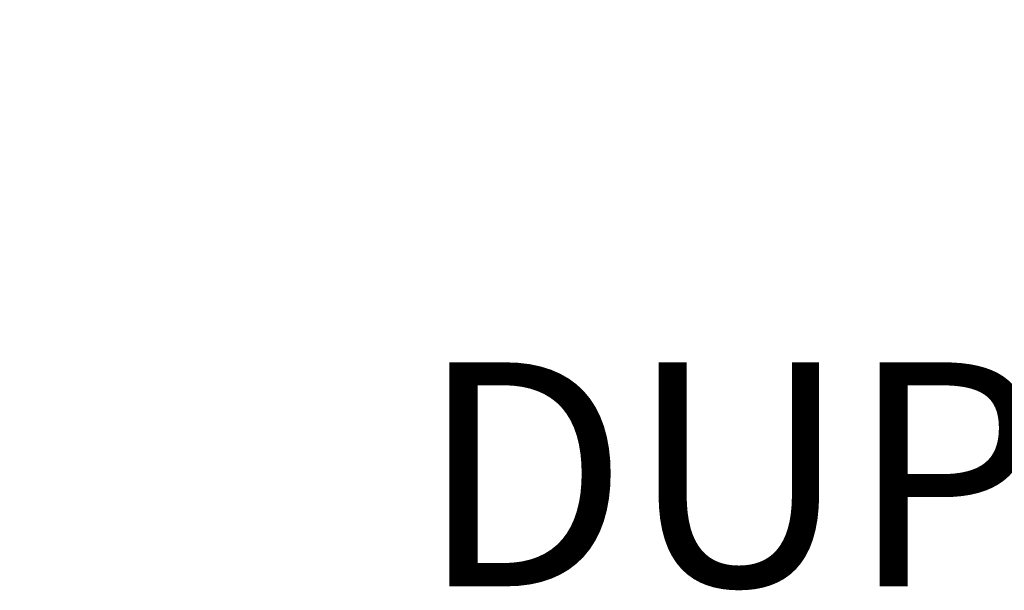
# Model space of a CAD drawing. Units: inches. Extents: x 351 to 1738, y -265 to 286.
# Tile 9 of 38: x 1074 to 1176, y -265 to -206. Entities that reach past the tile are written whole.
import ezdxf

# ---------------------------------------------------------------- set-up
doc = ezdxf.new("R2010")
doc.units = ezdxf.units.IN
doc.header["$MEASUREMENT"] = 0
doc.layers.add('A-ANNO-DIMS', color=2, linetype='Continuous', lineweight=18)
doc.layers.add('A-ANNO-TITL', color=7, linetype='Continuous', lineweight=35)
doc.styles.add('Annotative', font='arial.ttf')
doc.styles.get("Standard").update_dxf_attribs({"font": 'arial.ttf'})
doc.dimstyles.get("Standard").update_dxf_attribs({"dimtxt": 8, "dimasz": 5, "dimexe": 0.18, "dimexo": 0.0625, "dimgap": 0.09, "dimtad": 1, "dimtoh": 1, "dimzin": 0, "dimdsep": 46, "dimlunit": 4, "dimtxsty": 'Standard', "dimcen": 0, "dimclre": 256, "dimadec": 0, "dimazin": 0, "dimtfac": 1, "dimtofl": 0, "dimtmove": 0, "dimatfit": 3, "dimfxl": 1, "dimtolj": 1, "dimtzin": 0, "dimlwe": -1, "dimarcsym": 0})

# ---------------------------------------------------------------- blocks, each defined once
blk = doc.blocks.new('*D36')
at = {"layer": 'A-ANNO-DIMS', "transparency": 16777216}
for p, q in [((1073.57, -199.34), (1073.57, -204.2)), ((1105.2, -199.34), (1105.2, -204.2))]:
    blk.add_line(p, q, dxfattribs=at)
at = {"layer": 'A-ANNO-DIMS', "color": 0, "lineweight": -2, "transparency": 16777216}
for p, q in [((1078.57, -204.02), (1100.2, -204.02)), ((1105.2, -204.02), (1227.07, -204.02))]:
    blk.add_line(p, q, dxfattribs=at)
at = {"layer": 'A-ANNO-DIMS', "color": 0, "transparency": 16777216}
for points in [[(1078.57, -203.19), (1078.57, -204.86), (1073.57, -204.02)], [(1100.2, -203.19), (1100.2, -204.86), (1105.2, -204.02)]]:
    blk.add_solid(points, dxfattribs=at)
at = {"layer": 'Defpoints', "color": 0, "transparency": 16777216}
for p in [(1073.57, -199.28), (1105.2, -199.28), (1105.2, -204.02)]:
    blk.add_point(p, dxfattribs=at)
at = {"layer": 'A-ANNO-DIMS', "color": 0, "transparency": 16777216, "insert": (1168.63, -199.8), "char_height": 8, "attachment_point": 5}
blk.add_mtext('\\A1;PLANT A 2\'-7 1/2" TYP.', dxfattribs=at)

msp = doc.modelspace()

# ---------------------------------------------------------------- texts
at = {"layer": 'A-ANNO-TITL', "style": 'Annotative'}
msp.add_text('DUPLEX THIRD FLOOR', height=23.27476, dxfattribs=at).set_placement((1115.071, -264.89))

# ---------------------------------------------------------------- dimensions: what is measured, and where the dimension line sits
at = {"layer": 'A-ANNO-DIMS'}
dim = msp.add_linear_dim(base=(1105.198, -204.022), p1=(1073.569, -199.278), p2=(1105.198, -199.278), text='PLANT A <> TYP.', dimstyle='Standard', override={"dimdec": 1, "dimlfac": 1, "dimrnd": 0, "dimzin": 1, "dimdsep": 46, "dimlunit": 4, "dimfrac": 2}, dxfattribs=at)
dim.commit()
dim.dimension.update_dxf_attribs({"geometry": '*D36', "text_midpoint": (1168.634, -199.796)})

doc.saveas('drawing.dxf')
